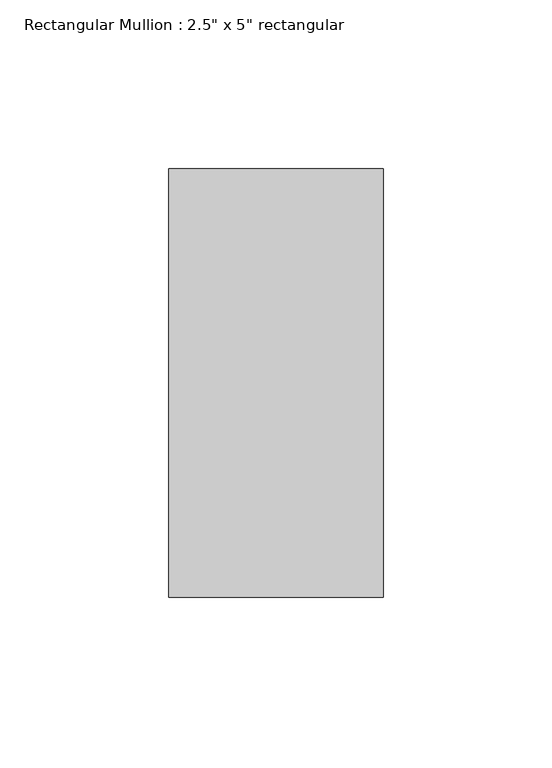
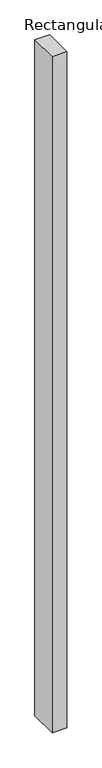
"""IFC4 building model written with IfcOpenShell, lengths in millimetres: member geometry."""

from ifc_helpers import new_model, si_unit, frame, origin, place, context, project, spatial, polyline, outline, extrude, source, transform, mapped, element, save


def member_a37e84cf(model_context):
    return source(origin(), model_context, "Body", "SweptSolid", [
        extrude(outline(polyline([(0.0, 63.5), (0.0, -63.5), (-63.5, -63.5), (-63.5, 63.5), (0.0, 63.5)])), frame((0.0, 0.0, -3052.9241767), z_axis=(0.0, 0.0, 1.0), x_axis=(1.0, 0.0, 0.0)), (0.0, 0.0, 1.0), 3052.9241767),
    ])


if __name__ == "__main__":
    model = new_model("IFC4")
    model_context = context("Model", 3, world=origin())
    ifc_project = project(units=[si_unit("LENGTHUNIT", "METRE", prefix="MILLI")], contexts=[model_context])
    site = spatial("IfcSite", under=ifc_project)
    building = spatial("IfcBuilding", under=site)
    placement = place(None, origin())
    member_shape = member_a37e84cf(model_context)
    element("IfcMember", 1, ObjectType="Rectangular Mullion : 2.5\" x 5\" rectangular", at=placement, inside=building, context=model_context, shape_type="MappedRepresentation", body=[
        mapped(member_shape, transform((0.0, 0.0, 0.0), x_axis=(1.0, 0.0, 0.0), y_axis=(0.0, 1.0, 0.0), z_axis=(0.0, 0.0, 1.0))),
    ])
    save(model, "model.ifc")

# Revit data of these elements
# Type "Rectangular Mullion : 2.5\" x 5\" rectangular"
#   built-in parameter 1007304 = 0.416667 (stored number, unit not read)
#   built-in parameter 1007301 = 0.104167 (stored number, unit not read)
#   built-in parameter 1007300 = 0.104167 (stored number, unit not read)
# Element 1 (IfcMember, "Rectangular Mullion : 2.5\" x 5\" rectangular")
#   Materials on its faces: "Aluminum"
# Materials
#   "Aluminum": class "Metal", colour RGB 247 247 247, transparency 0, Description = "Aluminum 6061", Cost = 0
